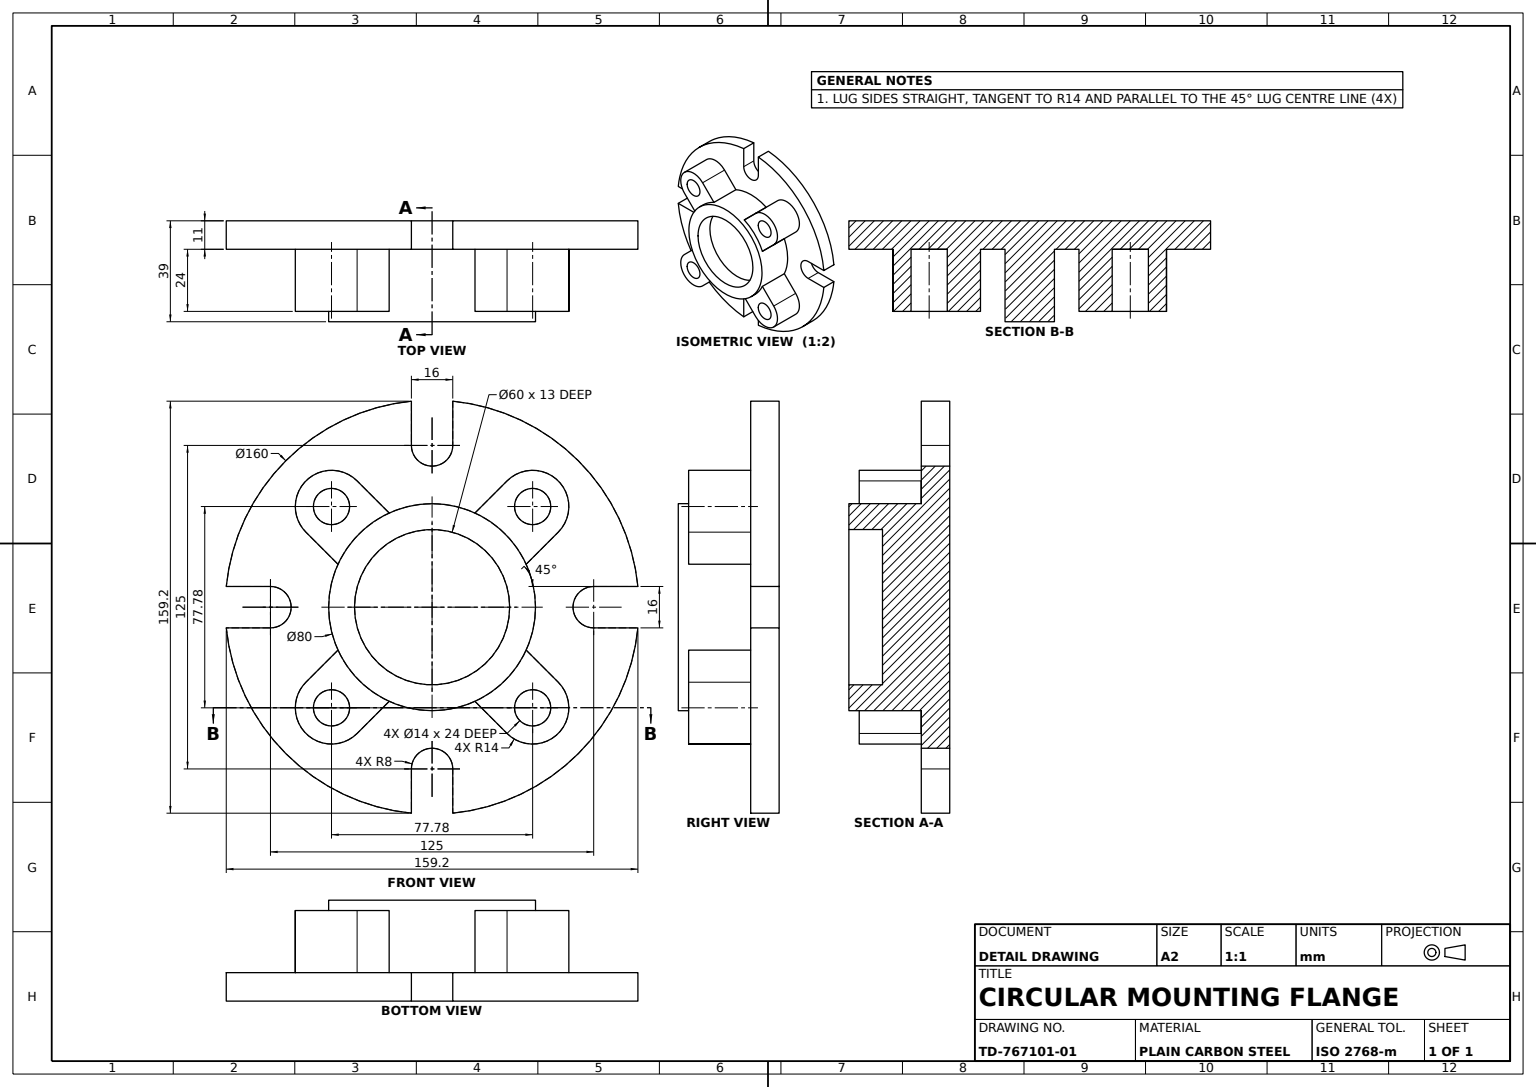
SolidWorks part; units mm, degrees
material "Plain Carbon Steel"
ref_plane "Front Plane" through (0, 0, 0) normal (0, 0, 1) x (1, 0, 0)
ref_plane "Top Plane" through (0, 0, 0) normal (0, 1, 0) x (1, 0, 0)
ref_plane "Right Plane" through (0, 0, 0) normal (1, 0, 0) x (0, 0, -1)
sketch "Flange Disc Sketch" plane through (0, 0, 0) normal (0, 0, 1) x (1, 0, 0)
  circle A0 centre (0, 0) radius 80
  dimension "D1" = 160
extrude "Flange Disc Ø160" add sketch "Flange Disc Sketch" along normal blind 11
sketch "Hub Sketch" plane through (0, 0, 11) normal (0, 0, 1) x (1, 0, 0)
  circle A0 centre (0, 0) radius 40
  circle A1 centre (0, 0) radius 30
  dimension "D1" = 80
  dimension "D2" = 60
extrude "Hub Ø80xØ60" add sketch "Hub Sketch" along normal blind 28
sketch "Round Boss Sketch" plane through (0, 0, 11) normal (0, 0, 1) x (1, 0, 0)
  circle A0 centre (0, 0) radius 30
  dimension "D1" = 60
extrude "Round Boss 15mm" add sketch "Round Boss Sketch" along normal blind 15
sketch "Mounting Lug Sketch" plane through (0, 0, 11) normal (0, 0, 1) x (1, 0, 0)
  line L0 (0, 0) -> (80, 0) construction
  line L1 (0, 0) -> (56.5685, 56.5685) construction
  line L7 (16.5958, 36.3948) -> (28.9914, 48.7904)
  line L8 (36.3948, 16.5958) -> (48.7904, 28.9914)
  circle A0 centre (0, 0) radius 55 construction
  circle A1 centre (0, 0) radius 80 construction
  arc A2 (48.7904, 28.9914) -> (28.9914, 48.7904) centre (38.8909, 38.8909) ccw
  arc A5 (36.3948, 16.5958) -> (16.5958, 36.3948) centre (0, 0) ccw
  circle A6 centre (38.8909, 38.8909) radius 7
  dimension "D1" = 110
  dimension "D3" = 14
  dimension "D5" = 14
  dimension "D4" = 14
  dimension "D6" = 40
  dimension "D2" = 45
extrude "Mounting Lug" add sketch "Mounting Lug Sketch" along normal blind 24
pattern_circular "Mounting Lug Pattern 4x" count 4 over 360 about axis through (0, 0, 0) along (0, 0, 1) of "Mounting Lug"
sketch "Rim Slot Sketch" plane through (0, 0, 11) normal (0, 0, 1) x (1, 0, 0)
  line L0 (0, 0) -> (62.5, 0) construction
  line L1 (62.5, 8) -> (79.599, 8)
  line L2 (62.5, -8) -> (79.599, -8)
  circle A0 centre (0, 0) radius 62.5 construction
  arc A1 (62.5, 8) -> (62.5, -8) centre (62.5, 0) ccw
  circle A2 centre (0, 0) radius 80 construction
  arc A3 (79.599, -8) -> (79.599, 8) centre (0, 0) ccw
  dimension "D1" = 125
  dimension "D2" = 8
extrude "Rim Slot Cut" cut sketch "Rim Slot Sketch" against normal blind 24
pattern_circular "Rim Slot Pattern 4x" count 4 over 360 about axis through (0, 0, 0) along (0, 0, 1) of "Rim Slot Cut"
